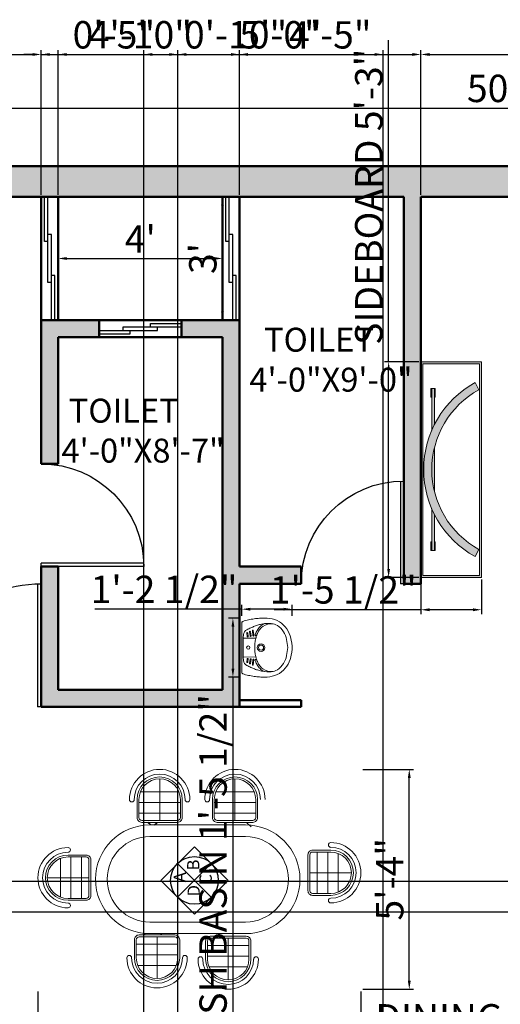
# Model space of a CAD drawing. Units: inches. Extents: x 1770 to 3141, y 984 to 1614.
# Tile 4 of 12: x 1974 to 2115, y 1320 to 1608. Entities that reach past the tile are written whole.
import ezdxf

# ---------------------------------------------------------------- set-up
doc = ezdxf.new("R2010")
doc.units = ezdxf.units.IN
for name, color, linetype, lineweight in [('0.15', 34, 'Continuous', 15), ('A-ANNO-DIMS', 2, 'Continuous', 18), ('A-AREA-IDEN', 3, 'Continuous', 18), ('A-DOOR', 4, 'Continuous', 25), ('A-FLOR-FIXT', 8, 'Continuous', 18), ('A-FURN', 8, 'Continuous', 18), ('A-GLAZ', 5, 'Continuous', 25), ('A-WALL', 7, 'Continuous', 50), ('A-WALL-PATT', 8, 'Continuous', 13), ('aparador', 36, 'Continuous', 9), ('moveis', 254, 'Continuous', 5)]:
    doc.layers.add(name, color=color, linetype=linetype, lineweight=lineweight)
doc.layers.add('4', color=4, linetype='Continuous')
doc.styles.get("Standard").update_dxf_attribs({"font": 'arial.ttf'})
doc.dimstyles.new('ISO-25', dxfattribs={"dimtxt": 8, "dimasz": 2.5, "dimexe": 1.25, "dimexo": 0.625, "dimtad": 1, "dimdec": 1, "dimlunit": 3, "dimtxsty": 'Standard', "dimcen": 2.5, "dimclrt": 1, "dimadec": 0, "dimazin": 0, "dimtfac": 1, "dimtdec": 1, "dimtmove": 0, "dimatfit": 3, "dimfxl": 1, "dimarcsym": 0})

# ---------------------------------------------------------------- blocks, each defined once
blk = doc.blocks.new("D1 3'")
for p, q in [((0, 36), (0, 0)), ((1, 36), (1, 0)), ((0, 0), (1, 0))]:
    blk.add_line(p, q)
blk.add_arc((0, 0), 36, 0, 90)
blk = doc.blocks.new("D2 2'6")
for p, q in [((0, 30), (0, 0)), ((1, 30), (1, 0)), ((0, 0), (1, 0))]:
    blk.add_line(p, q)
blk.add_arc((0, 0), 30, 0, 90)
blk = doc.blocks.new('*D17')
at = {"layer": 'A-ANNO-DIMS', "color": 0, "lineweight": -2, "transparency": 16777216}
for p, q in [((1812.73, 1565.8), (1812.73, 1583.37)), ((1815.23, 1582.12), (2410.23, 1582.12)), ((2412.73, 1565.8), (2412.73, 1583.37))]:
    blk.add_line(p, q, dxfattribs=at)
at = {"layer": 'A-ANNO-DIMS', "color": 0, "transparency": 16777216}
for points in [[(1815.23, 1582.54), (1815.23, 1581.7), (1812.73, 1582.12)], [(2410.23, 1582.54), (2410.23, 1581.7), (2412.73, 1582.12)]]:
    blk.add_solid(points, dxfattribs=at)
at = {"layer": 'Defpoints', "color": 0, "transparency": 16777216}
for p in [(2412.73, 1582.12), (1812.73, 1565.18), (2412.73, 1565.18)]:
    blk.add_point(p, dxfattribs=at)
at = {"layer": 'A-ANNO-DIMS', "color": 0, "transparency": 16777216, "insert": (2112.73, 1586.83), "char_height": 8, "attachment_point": 5}
blk.add_mtext("50'", dxfattribs=at)
blk = doc.blocks.new('A$C124A256F')
for p, q in [((-0.448, 1.309), (-0.448, 0.772)), ((0.523, 1.309), (0.523, 0.772)), ((-0.697, 1.141), (-0.2, 1.141)), ((0.772, 1.141), (0.275, 1.141)), ((-0.715, 1.006), (-0.181, 1.006)), ((0.791, 1.006), (0.256, 1.006)), ((-0.715, 0.867), (-0.181, 0.867)), ((0.791, 0.867), (0.256, 0.867)), ((-1.729, -0.214), (-1.729, 0.283)), ((-1.594, -0.233), (-1.594, 0.302)), ((-1.455, -0.233), (-1.455, 0.302)), ((1.583, -0.169), (1.583, 0.365)), ((1.721, -0.169), (1.721, 0.365)), ((1.856, -0.15), (1.856, 0.346)), ((-1.897, 0.034), (-1.361, 0.034)), ((2.025, 0.098), (1.488, 0.098)), ((-0.482, -1.265), (-0.482, -0.728)), ((0.436, -1.282), (0.436, -0.745)), ((-0.749, -0.823), (-0.215, -0.823)), ((0.704, -0.84), (0.169, -0.84)), ((-0.749, -0.962), (-0.215, -0.962)), ((0.704, -0.978), (0.169, -0.978)), ((-0.73, -1.097), (-0.233, -1.097)), ((0.685, -1.114), (0.188, -1.114))]:
    blk.add_line(p, q)
for points in [[(-0.217, 0.748), (-0.679, 0.748, -0.414214), (-0.74, 0.809), (-0.74, 1.042, -1), (-0.157, 1.042), (-0.157, 0.809, -0.414214)], [(-0.217, 0.772), (-0.679, 0.772, -0.414214), (-0.715, 0.809), (-0.715, 1.042, -1), (-0.181, 1.042), (-0.181, 0.809, -0.414214)], [(0.293, 0.748), (0.754, 0.748, 0.414214), (0.815, 0.809), (0.815, 1.042, 1), (0.232, 1.042), (0.232, 0.809, 0.414214)], [(0.293, 0.772), (0.754, 0.772, 0.414214), (0.791, 0.809), (0.791, 1.042, 1), (0.256, 1.042), (0.256, 0.809, 0.414214)], [(1.464, 0.329), (1.464, -0.133, 0.414214), (1.525, -0.194), (1.758, -0.194, 1), (1.758, 0.39), (1.525, 0.39, 0.414214)], [(-1.336, 0.265), (-1.336, -0.196, -0.414214), (-1.397, -0.257), (-1.63, -0.257, -1), (-1.63, 0.326), (-1.397, 0.326, -0.414214)], [(-1.361, 0.265), (-1.361, -0.196, -0.414214), (-1.397, -0.233), (-1.63, -0.233, -1), (-1.63, 0.302), (-1.397, 0.302, -0.414214)], [(1.488, 0.329), (1.488, -0.133, 0.414214), (1.525, -0.169), (1.758, -0.169, 1), (1.758, 0.365), (1.525, 0.365, 0.414214)], [(-0.251, -0.704), (-0.713, -0.704, 0.414214), (-0.774, -0.765), (-0.774, -0.998, 1), (-0.19, -0.998), (-0.19, -0.765, 0.414214)], [(-0.251, -0.728), (-0.713, -0.728, 0.414214), (-0.749, -0.765), (-0.749, -0.998, 1), (-0.215, -0.998), (-0.215, -0.765, 0.414214)], [(0.205, -0.721), (0.667, -0.721, -0.414214), (0.728, -0.782), (0.728, -1.015, -1), (0.145, -1.015), (0.145, -0.782, -0.414214)], [(0.205, -0.745), (0.667, -0.745, -0.414214), (0.704, -0.782), (0.704, -1.015, -1), (0.169, -1.015), (0.169, -0.782, -0.414214)]]:
    blk.add_lwpolyline(points, format="xyb", close=True)
for points in [[(-0.026, 0.714), (-0.575, 0.714, 1), (-0.575, -0.687), (-0.026, -0.687)], [(-0.026, -0.687), (0.661, -0.687, 1), (0.661, 0.714), (-0.026, 0.714)], [(0.254, 0.564), (-0.575, 0.564, 1), (-0.575, -0.537), (0.306, -0.537)], [(0.306, -0.537), (0.661, -0.537, 1), (0.661, 0.564), (0.254, 0.564)]]:
    blk.add_lwpolyline(points, format="xyb")
for centre, radius, start, end in [((-0.448, 1.042), 0.389, 0, 180), ((0.523, 1.042), 0.389, 0, 180), ((-0.448, 1.042), 0.328, 0, 180), ((0.523, 1.042), 0.328, 0, 180), ((-0.807, 1.042), 0.0304, 180, 0), ((-0.09, 1.042), 0.0304, 180, 0), ((0.165, 1.042), 0.0304, 180, 0), ((-1.63, 0.034), 0.389, 90, 270), ((-1.63, 0.393), 0.0304, 270, 90), ((1.758, 0.456), 0.0304, 90, 270), ((1.758, 0.098), 0.389, 270, 90), ((1.758, 0.098), 0.328, 270, 90), ((-1.63, 0.034), 0.328, 90, 270), ((1.758, -0.26), 0.0304, 90, 270), ((-1.63, -0.324), 0.0304, 270, 90), ((-0.84, -0.998), 0.0304, 0, 180), ((-0.482, -0.998), 0.389, 180, 0), ((-0.482, -0.998), 0.328, 180, 0), ((-0.123, -0.998), 0.0304, 0, 180), ((0.078, -1.015), 0.0304, 0, 180), ((0.436, -1.015), 0.389, 180, 0), ((0.436, -1.015), 0.328, 180, 0), ((0.795, -1.015), 0.0304, 0, 180)]:
    blk.add_arc(centre, radius, start, end)
at = {"layer": '4'}
for p, q in [((-0.566, 0.714), (-0.6, 0.748)), ((-0.513, 0.714), (-0.479, 0.748)), ((0.733, 0.688), (0.673, 0.748)), ((-0.217, -0.217), (0.217, 0.217)), ((-0.217, 0.217), (0.217, -0.217)), ((-0.659, -0.704), (-0.638, -0.684)), ((-0.421, -0.704), (-0.438, -0.687))]:
    blk.add_line(p, q, dxfattribs=at)
blk.add_lwpolyline([(0, -0.434), (-0.434, 0), (0, 0.434), (0.434, 0)], close=True, dxfattribs=at)
blk.add_circle((0, 0), 0.307, dxfattribs=at)
for s, height, p in [('B', 0.158, (0.064, 0.127)), ('A ', 0.1575, (-0.109, -0.025)), ('C', 0.158, (0.224, -0.057)), ('D', 0.158, (0.07, -0.208))]:
    blk.add_text(s, height=height, rotation=90, dxfattribs=at).set_placement(p)
blk = doc.blocks.new('Aparador ORGANICA Formatto')
at = {"layer": 'aparador', "ltscale": 0.3}
h = blk.add_hatch(color=256, dxfattribs=at)
h.dxf.hatch_style = 1
h.set_gradient(color1=(118, 213, 123), color2=(52, 168, 57), one_color=1, tint=0.43, name='INVCURVED')
h.paths.add_polyline_path([(0.8, 0.45), (-0.8, 0.45), (-0.8, 0), (0.8, 0)])
h.paths.add_polyline_path([(0.785, 0.435), (0.785, 0.015), (-0.785, 0.015), (-0.785, 0.435)], flags=16)
h.paths.add_polyline_path([(0.2911, 0.3699), (0.5365, 0.3699), (0.5365, 0.3757), (0.6011, 0.3757), (0.6011, 0.3699), (0.6011, 0.3499), (0.6011, 0.3441), (0.5365, 0.3441), (0.5365, 0.3499), (0.3338, 0.3499, -0.150336), (0.6449, 0.0488), (0.5923, 0.0199, 0.208852), (0.1632, 0.3499), (-0.1632, 0.3499, 0.208852), (-0.5923, 0.0199), (-0.6449, 0.0488, -0.150336), (-0.3338, 0.3499), (-0.5365, 0.3499), (-0.5365, 0.3441), (-0.6011, 0.3441), (-0.6011, 0.3499), (-0.6011, 0.3699), (-0.6011, 0.3757), (-0.5365, 0.3757), (-0.5365, 0.3699), (-0.2911, 0.3699, -0.206106)], flags=0)
h = blk.add_hatch(color=256, dxfattribs=at)
h.dxf.hatch_style = 1
h.set_gradient(color1=(135, 92, 69), color2=(0, 0, 0), one_color=1, name='INVCURVED')
h.paths.add_polyline_path([(-0.6449, 0.0488), (-0.5923, 0.0199, -0.590888), (0.5923, 0.0199), (0.6449, 0.0488, 0.590888)])
h = blk.add_hatch(color=256, dxfattribs=at)
h.dxf.hatch_style = 1
h.set_gradient(color1=(178, 189, 189), one_color=1, tint=1, name='CYLINDER')
h.paths.add_polyline_path([(-0.5365, 0.3757), (-0.6011, 0.3757), (-0.6011, 0.3699), (-0.5365, 0.3699)])
h.paths.add_polyline_path([(-0.5365, 0.3499), (-0.6011, 0.3499), (-0.6011, 0.3441), (-0.5365, 0.3441)])
h = blk.add_hatch(color=256, dxfattribs=at)
h.dxf.hatch_style = 1
h.set_gradient(color1=(118, 213, 123), color2=(31, 101, 35), one_color=1, tint=0.26, name='INVCURVED')
h.paths.add_polyline_path([(-0.2911, 0.3699), (-0.6011, 0.3699), (-0.6011, 0.3499), (-0.3338, 0.3499, -0.015999)])
h = blk.add_hatch(color=256, dxfattribs=at)
h.dxf.hatch_style = 1
h.set_gradient(color1=(118, 213, 123), color2=(31, 101, 35), one_color=1, tint=0.26, name='INVCURVED')
h.paths.add_polyline_path([(-0.1632, 0.3499), (0.1632, 0.3499, 0.122516)])
h = blk.add_hatch(color=256, dxfattribs=at)
h.dxf.hatch_style = 1
h.set_gradient(color1=(118, 213, 123), color2=(31, 101, 35), one_color=1, tint=0.26, name='INVCURVED')
h.paths.add_polyline_path([(0.6011, 0.3699), (0.2911, 0.3699, -0.015999), (0.3338, 0.3499), (0.6011, 0.3499)])
h = blk.add_hatch(color=256, dxfattribs=at)
h.dxf.hatch_style = 1
h.set_gradient(color1=(178, 189, 189), one_color=1, tint=1, name='CYLINDER')
h.paths.add_polyline_path([(0.6011, 0.3757), (0.5365, 0.3757), (0.5365, 0.3699), (0.6011, 0.3699)])
h.paths.add_polyline_path([(0.6011, 0.3499), (0.5365, 0.3499), (0.5365, 0.3441), (0.6011, 0.3441)])
for p, q in [((-0.5923, 0.0199), (-0.6449, 0.0488)), ((0.5923, 0.0199), (0.6449, 0.0488))]:
    blk.add_line(p, q, dxfattribs=at)
for points in [[(-0.6011, 0.3699), (-0.6011, 0.3757), (-0.5365, 0.3757), (-0.5365, 0.3699)], [(0.6011, 0.3699), (0.6011, 0.3757), (0.5365, 0.3757), (0.5365, 0.3699)], [(-0.5365, 0.3499), (-0.5365, 0.3441), (-0.6011, 0.3441), (-0.6011, 0.3499)], [(0.5365, 0.3499), (0.5365, 0.3441), (0.6011, 0.3441), (0.6011, 0.3499)]]:
    blk.add_lwpolyline(points, dxfattribs=at)
for radius in [0.7362, 0.6762]:
    blk.add_arc((0, -0.3063), radius, 28.84335, 151.15665, dxfattribs=at)
at = {"layer": 'moveis', "ltscale": 0.3}
for p, q in [((-0.6011, 0.3699), (-0.6011, 0.3499)), ((-0.2911, 0.3699), (-0.6011, 0.3699)), ((0.2911, 0.3699), (0.6011, 0.3699)), ((0.6011, 0.3699), (0.6011, 0.3499)), ((-0.6011, 0.3499), (-0.3338, 0.3499)), ((-0.1632, 0.3499), (0.1632, 0.3499)), ((0.6011, 0.3499), (0.3338, 0.3499))]:
    blk.add_line(p, q, dxfattribs=at)
for points in [[(-0.8, 0), (0.8, 0), (0.8, 0.45), (-0.8, 0.45)], [(-0.785, 0.015), (0.785, 0.015), (0.785, 0.435), (-0.785, 0.435)]]:
    blk.add_lwpolyline(points, close=True, dxfattribs=at)
blk = doc.blocks.new('*D56')
at = {"layer": 'A-ANNO-DIMS', "color": 0, "lineweight": -2, "transparency": 16777216}
for p, q in [((1985.73, 1538.8), (1985.73, 1539.43)), ((2033.73, 1538.8), (2033.73, 1539.43)), ((1988.23, 1538.18), (2031.23, 1538.18))]:
    blk.add_line(p, q, dxfattribs=at)
at = {"layer": 'A-ANNO-DIMS', "color": 0, "transparency": 16777216}
for points in [[(1988.23, 1538.6), (1988.23, 1537.76), (1985.73, 1538.18)], [(2031.23, 1538.6), (2031.23, 1537.76), (2033.73, 1538.18)]]:
    blk.add_solid(points, dxfattribs=at)
at = {"layer": 'Defpoints', "color": 0, "transparency": 16777216}
for p in [(1985.73, 1538.18), (2033.73, 1538.18), (2033.73, 1538.18)]:
    blk.add_point(p, dxfattribs=at)
at = {"layer": 'A-ANNO-DIMS', "color": 0, "transparency": 16777216, "insert": (2009.73, 1542.8), "char_height": 8, "attachment_point": 5}
blk.add_mtext("4'", dxfattribs=at)
blk = doc.blocks.new('*D57')
at = {"layer": 'A-ANNO-DIMS', "color": 0, "lineweight": -2, "transparency": 16777216}
for p, q in [((2028.55, 1556.18), (2034.98, 1556.18)), ((2033.73, 1553.68), (2033.73, 1522.68)), ((2028.55, 1520.18), (2034.98, 1520.18))]:
    blk.add_line(p, q, dxfattribs=at)
at = {"layer": 'A-ANNO-DIMS', "color": 0, "transparency": 16777216}
for points in [[(2033.32, 1553.68), (2034.15, 1553.68), (2033.73, 1556.18)], [(2033.32, 1522.68), (2034.15, 1522.68), (2033.73, 1520.18)]]:
    blk.add_solid(points, dxfattribs=at)
at = {"layer": 'Defpoints', "color": 0, "transparency": 16777216}
for p in [(2027.93, 1556.18), (2027.93, 1520.18), (2033.73, 1520.18)]:
    blk.add_point(p, dxfattribs=at)
at = {"layer": 'A-ANNO-DIMS', "color": 0, "transparency": 16777216, "insert": (2029.02, 1538.18), "char_height": 8, "attachment_point": 5, "rotation": 90}
blk.add_mtext("3'", dxfattribs=at)
blk = doc.blocks.new('lavamanos 2')
at = {"layer": '0.15'}
for p, q in [((0, 0.2335), (0, -0.2335)), ((-0.1304, 0.11), (-0.1315, 0.11)), ((-0.1127, 0.112), (-0.1067, 0.1581)), ((-0.1037, 0.1109), (-0.0978, 0.157)), ((-0.0857, 0.1085), (-0.0807, 0.1466)), ((-0.0767, 0.1074), (-0.0718, 0.1455)), ((-0.0587, 0.105), (-0.0548, 0.1351)), ((-0.0497, 0.1039), (-0.0458, 0.134)), ((-0.0142, 0.087), (-0.13, 0.086)), ((-0.0142, -0.087), (-0.13, -0.086)), ((-0.1304, -0.11), (-0.1315, -0.11)), ((-0.1127, -0.112), (-0.1067, -0.1581)), ((-0.1037, -0.1109), (-0.0978, -0.157)), ((-0.0857, -0.1085), (-0.0807, -0.1466)), ((-0.0767, -0.1074), (-0.0718, -0.1455)), ((-0.0587, -0.105), (-0.0548, -0.1351)), ((-0.0497, -0.1039), (-0.0458, -0.134))]:
    blk.add_line(p, q, dxfattribs=at)
for centre, radius in [((-0.178, 0), 0.035), ((-0.178, 0), 0.0235), ((-0.06, 0), 0.015)]:
    blk.add_circle(centre, radius, dxfattribs=at)
for centre, radius, start, end in [((-0.2035, -0.0862), 0.3593, 91.20299, 106.42552), ((-0.2208, -0.6855), 0.9585, 86.55138, 89.41308), ((-0.1663, 0.0005), 0.3024, 136.57187, 154.32772), ((-0.2419, 0.0663), 0.2023, 108.1945, 135.36859), ((-0.2422, 0.0655), 0.1638, 121.99295, 150.58892), ((-0.2657, 0.1037), 0.119, 92.47742, 122.14108), ((-0.2765, 0.0677), 0.1528, 57.2491, 95.54005), ((-0.2442, -0.0128), 0.2368, 77.24819, 96.46321), ((-0.2765, 0.0677), 0.1678, 56.87663, 64.99714), ((-0.3662, -0.002), 0.2627, 40.35252, 49.00458), ((-0.2222, 0.0026), 0.2177, 71.98488, 82.01242), ((-0.3662, -0.002), 0.2777, 40.35252, 49.22548), ((-0.2121, -0.5476), 0.8204, 83.12241, 86.5796), ((-0.3103, -0.315), 0.5472, 69.51913, 73.49118), ((-0.2991, -0.2855), 0.5156, 65.23004, 69.53785), ((5.8279, 30.215), 30.5319, 258.77821, 258.87599), ((-0.2784, -0.2408), 0.4663, 60.24131, 65.2382), ((-0.1265, -0.0657), 0.3287, 69.06009, 78.82181), ((-0.0202, 0.212), 0.0314, 54.79491, 69.06009), ((-0.005, 0.2335), 0.005, 0, 54.79491), ((-0.0557, -0.0178), 0.4111, 158.70106, 171.31016), ((-0.1999, 0.0263), 0.2202, 147.11565, 167.44248), ((-0.2374, 0.11), 0.0921, 27.31862, 39.11562), ((-0.3494, 0.0363), 0.2258, 22.33605, 30.8927), ((-0.2374, 0.11), 0.1071, 27.57433, 39.11562), ((-0.3494, 0.0363), 0.2408, 22.19214, 30.78376), ((-1.2664, -0.2389), 1.1824, 16.36313, 17.77674), ((-0.1315, 0.117), 0.007, 197.40991, 270.49494), ((0.1853, 0.1648), 0.325, 192.53887, 196.70718), ((-0.1305, 0.117), 0.007, 270.49494, 17.39527), ((-1.2664, -0.2389), 1.1974, 17.39527, 17.80495), ((-0.1082, 0.1115), 0.0045, 172.61396, 352.61396), ((-0.1022, 0.1575), 0.0045, 352.61396, 172.61396), ((-0.0812, 0.108), 0.0045, 172.61396, 352.61396), ((-0.0763, 0.146), 0.0045, 352.61396, 172.61396), ((-0.0542, 0.1045), 0.0045, 172.61396, 352.61396), ((-0.0503, 0.1345), 0.0045, 352.61396, 172.61396), ((-0.0648, 0.1184), 0.049, 1.58272, 68.62081), ((-2.1477, 0.0009), 2.1352, 359.97535, 3.19009), ((-0.2093, 0.0056), 0.2558, 171.31016, 181.26266), ((-0.2093, -0.0056), 0.2558, 178.73734, 188.68984), ((0.4664, -0.0834), 0.8953, 169.86317, 174.65802), ((0.4664, 0.0834), 0.8953, 185.34198, 190.13683), ((0.3887, 0.121), 0.517, 185.50529, 189.81306), ((-0.7181, -0.0071), 0.5987, 0.67647, 3.82165), ((-0.7181, 0.0071), 0.5987, 356.17835, 359.32353), ((-2.1477, -0.0009), 2.1352, 356.80991, 0.02465), ((-0.0557, 0.0178), 0.4111, 188.68984, 201.29894), ((-0.1999, -0.0263), 0.2202, 192.55752, 212.88435), ((0.1853, -0.1648), 0.325, 163.29282, 167.46113), ((0.3887, -0.1209), 0.517, 170.18694, 174.49471), ((-0.1663, -0.0005), 0.3024, 205.67228, 223.42813), ((-0.2422, -0.0655), 0.1638, 209.41108, 238.00705), ((-0.3662, 0.002), 0.2627, 310.99542, 319.64748), ((-0.3662, 0.002), 0.2777, 310.77452, 319.64748), ((-0.2374, -0.1099), 0.0921, 320.88438, 332.68138), ((-0.3494, -0.0363), 0.2258, 329.1073, 337.66395), ((-0.2374, -0.1099), 0.1071, 320.88438, 332.42567), ((-0.3494, -0.0363), 0.2408, 329.21624, 337.80786), ((-1.2664, 0.2389), 1.1824, 342.22326, 343.63687), ((-0.1315, -0.117), 0.007, 89.50506, 162.59009), ((-0.1305, -0.117), 0.007, 342.60473, 89.50506), ((-1.2664, 0.2389), 1.1974, 342.19505, 342.60473), ((-0.1082, -0.1115), 0.0045, 7.38604, 187.38604), ((-0.1022, -0.1575), 0.0045, 187.38604, 7.38604), ((-0.0812, -0.108), 0.0045, 7.38604, 187.38604), ((-0.2784, 0.2408), 0.4663, 294.7618, 299.75869), ((-0.0763, -0.146), 0.0045, 187.38604, 7.38604), ((-0.0542, -0.1045), 0.0045, 7.38604, 187.38604), ((-0.0503, -0.1345), 0.0045, 187.38604, 7.38604), ((-0.0648, -0.1184), 0.049, 291.37919, 358.41728), ((-0.2419, -0.0663), 0.2023, 224.63141, 251.8055), ((-0.2657, -0.1036), 0.119, 237.85892, 267.52258), ((-0.2035, 0.0862), 0.3593, 253.57448, 268.79701), ((-0.2765, -0.0677), 0.1528, 264.45995, 302.7509), ((-0.2442, 0.0128), 0.2368, 263.53679, 282.75181), ((-0.2208, 0.6855), 0.9585, 270.58692, 273.44862), ((-0.2765, -0.0677), 0.1678, 295.00286, 303.12337), ((-0.2222, -0.0026), 0.2177, 277.98758, 288.01512), ((-0.2121, 0.5476), 0.8204, 273.4204, 276.87759), ((-0.3103, 0.315), 0.5472, 286.50882, 290.48087), ((-0.2991, 0.2855), 0.5156, 290.46215, 294.76996), ((5.8279, -30.215), 30.5319, 101.12401, 101.22179), ((-0.1265, 0.0657), 0.3287, 281.17819, 290.93991), ((-0.0202, -0.212), 0.0314, 290.93991, 305.20509), ((-0.005, -0.2335), 0.005, 305.20509, 0)]:
    blk.add_arc(centre, radius, start, end, dxfattribs=at)
blk = doc.blocks.new('*D92')
at = {"layer": 'A-ANNO-DIMS', "color": 0, "lineweight": -2, "transparency": 16777216}
for p, q in [((1979.79, 1324.09), (1979.79, 1309.31)), ((2074.16, 1324.09), (2074.16, 1309.31)), ((1982.29, 1310.56), (2071.66, 1310.56)), ((2074.16, 1310.56), (2190.7, 1310.56))]:
    blk.add_line(p, q, dxfattribs=at)
at = {"layer": 'A-ANNO-DIMS', "color": 0, "transparency": 16777216}
for points in [[(1982.29, 1310.98), (1982.29, 1310.15), (1979.79, 1310.56)], [(2071.66, 1310.98), (2071.66, 1310.15), (2074.16, 1310.56)]]:
    blk.add_solid(points, dxfattribs=at)
at = {"layer": 'Defpoints', "color": 0, "transparency": 16777216}
for p in [(1979.79, 1324.72), (2074.16, 1324.72), (2074.16, 1310.56)]:
    blk.add_point(p, dxfattribs=at)
at = {"layer": 'A-ANNO-DIMS', "color": 1, "transparency": 16777216, "insert": (2133.68, 1315.32), "char_height": 8, "attachment_point": 5}
blk.add_mtext('DINING SET 7\'-10 1/2"', dxfattribs=at)
blk = doc.blocks.new('*D93')
at = {"layer": 'A-ANNO-DIMS', "color": 0, "lineweight": -2, "transparency": 16777216}
for p, q in [((2074.79, 1388.94), (2089.57, 1388.94)), ((2088.32, 1327.22), (2088.32, 1386.44)), ((2074.79, 1324.72), (2089.57, 1324.72))]:
    blk.add_line(p, q, dxfattribs=at)
at = {"layer": 'A-ANNO-DIMS', "color": 0, "transparency": 16777216}
for points in [[(2087.9, 1386.44), (2088.74, 1386.44), (2088.32, 1388.94)], [(2087.9, 1327.22), (2088.74, 1327.22), (2088.32, 1324.72)]]:
    blk.add_solid(points, dxfattribs=at)
at = {"layer": 'Defpoints', "color": 0, "transparency": 16777216}
for p in [(2074.16, 1388.94), (2088.32, 1388.94), (2074.16, 1324.72)]:
    blk.add_point(p, dxfattribs=at)
at = {"layer": 'A-ANNO-DIMS', "color": 1, "transparency": 16777216, "insert": (2083.63, 1356.83), "char_height": 8, "attachment_point": 5, "rotation": 90}
blk.add_mtext('5\'-4"', dxfattribs=at)
blk = doc.blocks.new('*D96')
at = {"layer": 'A-ANNO-DIMS', "color": 0, "lineweight": -2, "transparency": 16777216}
for p, q in [((2082.28, 1508.01), (2082.28, 1601.92)), ((2091.11, 1508.01), (2081.03, 1508.01)), ((2082.28, 1447.52), (2082.28, 1505.51)), ((2091.11, 1445.02), (2081.03, 1445.02))]:
    blk.add_line(p, q, dxfattribs=at)
at = {"layer": 'A-ANNO-DIMS', "color": 0, "transparency": 16777216}
for points in [[(2081.87, 1505.51), (2082.7, 1505.51), (2082.28, 1508.01)], [(2081.87, 1447.52), (2082.7, 1447.52), (2082.28, 1445.02)]]:
    blk.add_solid(points, dxfattribs=at)
at = {"layer": 'Defpoints', "color": 0, "transparency": 16777216}
for p in [(2082.28, 1508.01), (2091.73, 1508.01), (2091.73, 1445.02)]:
    blk.add_point(p, dxfattribs=at)
at = {"layer": 'A-ANNO-DIMS', "color": 1, "transparency": 16777216, "insert": (2077.52, 1556.22), "char_height": 8, "attachment_point": 5, "rotation": 90}
blk.add_mtext('SIDEBOARD 5\'-3"', dxfattribs=at)
blk = doc.blocks.new('*D97')
at = {"layer": 'A-ANNO-DIMS', "color": 0, "lineweight": -2, "transparency": 16777216}
for p, q in [((2091.73, 1444.39), (2091.73, 1434.32)), ((2109.45, 1444.39), (2109.45, 1434.32)), ((2091.73, 1435.57), (2048.83, 1435.57)), ((2106.95, 1435.57), (2094.23, 1435.57))]:
    blk.add_line(p, q, dxfattribs=at)
at = {"layer": 'A-ANNO-DIMS', "color": 0, "transparency": 16777216}
for points in [[(2094.23, 1435.99), (2094.23, 1435.15), (2091.73, 1435.57)], [(2106.95, 1435.99), (2106.95, 1435.15), (2109.45, 1435.57)]]:
    blk.add_solid(points, dxfattribs=at)
at = {"layer": 'Defpoints', "color": 0, "transparency": 16777216}
for p in [(2091.73, 1445.02), (2109.45, 1445.02), (2091.73, 1435.57)]:
    blk.add_point(p, dxfattribs=at)
at = {"layer": 'A-ANNO-DIMS', "color": 1, "transparency": 16777216, "insert": (2069.03, 1440.33), "char_height": 8, "attachment_point": 5}
blk.add_mtext('1\'-5 1/2"', dxfattribs=at)
blk = doc.blocks.new('*D98')
at = {"layer": 'A-ANNO-DIMS', "color": 0, "lineweight": -2, "transparency": 16777216}
for p, q in [((2038.75, 1433.14), (2035.53, 1433.14)), ((2036.78, 1430.64), (2036.78, 1418.38)), ((2038.75, 1415.88), (2035.53, 1415.88)), ((2036.78, 1415.88), (2036.78, 1298.62))]:
    blk.add_line(p, q, dxfattribs=at)
at = {"layer": 'A-ANNO-DIMS', "color": 0, "transparency": 16777216}
for points in [[(2036.37, 1430.64), (2037.2, 1430.64), (2036.78, 1433.14)], [(2036.37, 1418.38), (2037.2, 1418.38), (2036.78, 1415.88)]]:
    blk.add_solid(points, dxfattribs=at)
at = {"layer": 'Defpoints', "color": 0, "transparency": 16777216}
for p in [(2039.37, 1433.14), (2036.78, 1415.88), (2039.37, 1415.88)]:
    blk.add_point(p, dxfattribs=at)
at = {"layer": 'A-ANNO-DIMS', "color": 1, "transparency": 16777216, "insert": (2032.02, 1356), "char_height": 8, "attachment_point": 5, "rotation": 89.9999}
blk.add_mtext('WASH BASIN 1\'-5 1/2"', dxfattribs=at)
blk = doc.blocks.new('*D99')
at = {"layer": 'A-ANNO-DIMS', "color": 0, "lineweight": -2, "transparency": 16777216}
for p, q in [((2039.37, 1435.73), (1996.47, 1435.73)), ((2039.37, 1433.76), (2039.37, 1436.98)), ((2051.58, 1435.73), (2041.87, 1435.73)), ((2054.08, 1433.76), (2054.08, 1436.98))]:
    blk.add_line(p, q, dxfattribs=at)
at = {"layer": 'A-ANNO-DIMS', "color": 0, "transparency": 16777216}
for points in [[(2041.87, 1436.15), (2041.87, 1435.31), (2039.37, 1435.73)], [(2051.58, 1436.15), (2051.58, 1435.31), (2054.08, 1435.73)]]:
    blk.add_solid(points, dxfattribs=at)
at = {"layer": 'Defpoints', "color": 0, "transparency": 16777216}
for p in [(2039.37, 1435.73), (2039.37, 1433.14), (2054.08, 1433.14)]:
    blk.add_point(p, dxfattribs=at)
at = {"layer": 'A-ANNO-DIMS', "color": 1, "transparency": 16777216, "insert": (2016.67, 1440.49), "char_height": 8, "attachment_point": 5, "rotation": 359.9999}
blk.add_mtext('1\'-2 1/2"', dxfattribs=at)
blk = doc.blocks.new('*D100')
at = {"layer": 'A-ANNO-DIMS', "color": 0, "lineweight": -2, "transparency": 16777216}
for p, q in [((1812.73, 1565.8), (1812.73, 1599.03)), ((1815.23, 1597.78), (1978.23, 1597.78)), ((1980.73, 1556.8), (1980.73, 1599.03))]:
    blk.add_line(p, q, dxfattribs=at)
at = {"layer": 'A-ANNO-DIMS', "color": 0, "transparency": 16777216}
for points in [[(1815.23, 1598.2), (1815.23, 1597.36), (1812.73, 1597.78)], [(1978.23, 1598.2), (1978.23, 1597.36), (1980.73, 1597.78)]]:
    blk.add_solid(points, dxfattribs=at)
at = {"layer": 'Defpoints', "color": 0, "transparency": 16777216}
for p in [(1980.73, 1597.78), (1812.73, 1565.18), (1980.73, 1556.18)]:
    blk.add_point(p, dxfattribs=at)
at = {"layer": 'A-ANNO-DIMS', "color": 1, "transparency": 16777216, "insert": (1896.73, 1602.49), "char_height": 8, "attachment_point": 5}
blk.add_mtext('14\'-0"', dxfattribs=at)
blk = doc.blocks.new('*D101')
at = {"layer": 'A-ANNO-DIMS', "color": 0, "lineweight": -2, "transparency": 16777216}
for p, q in [((1980.73, 1556.8), (1980.73, 1599.03)), ((1983.23, 1597.78), (2036.23, 1597.78)), ((2038.73, 1556.8), (2038.73, 1599.03))]:
    blk.add_line(p, q, dxfattribs=at)
at = {"layer": 'A-ANNO-DIMS', "color": 0, "transparency": 16777216}
for points in [[(1983.23, 1598.2), (1983.23, 1597.36), (1980.73, 1597.78)], [(2036.23, 1598.2), (2036.23, 1597.36), (2038.73, 1597.78)]]:
    blk.add_solid(points, dxfattribs=at)
at = {"layer": 'Defpoints', "color": 0, "transparency": 16777216}
for p in [(2038.73, 1597.78), (1980.73, 1556.18), (2038.73, 1556.18)]:
    blk.add_point(p, dxfattribs=at)
at = {"layer": 'A-ANNO-DIMS', "color": 1, "transparency": 16777216, "insert": (2009.73, 1602.49), "char_height": 8, "attachment_point": 5}
blk.add_mtext('4\'-10"', dxfattribs=at)
blk = doc.blocks.new('*D102')
at = {"layer": 'A-ANNO-DIMS', "color": 0, "lineweight": -2, "transparency": 16777216}
for p, q in [((2038.73, 1556.8), (2038.73, 1599.03)), ((2041.23, 1597.78), (2089.23, 1597.78)), ((2091.73, 1556.8), (2091.73, 1599.03))]:
    blk.add_line(p, q, dxfattribs=at)
at = {"layer": 'A-ANNO-DIMS', "color": 0, "transparency": 16777216}
for points in [[(2041.23, 1598.2), (2041.23, 1597.36), (2038.73, 1597.78)], [(2089.23, 1598.2), (2089.23, 1597.36), (2091.73, 1597.78)]]:
    blk.add_solid(points, dxfattribs=at)
at = {"layer": 'Defpoints', "color": 0, "transparency": 16777216}
for p in [(2091.73, 1597.78), (2038.73, 1556.18), (2091.73, 1556.18)]:
    blk.add_point(p, dxfattribs=at)
at = {"layer": 'A-ANNO-DIMS', "color": 1, "transparency": 16777216, "insert": (2065.23, 1602.47), "char_height": 8, "attachment_point": 5}
blk.add_mtext('4\'-5"', dxfattribs=at)
blk = doc.blocks.new('*D103')
at = {"layer": 'A-ANNO-DIMS', "color": 0, "lineweight": -2, "transparency": 16777216}
for p, q in [((2091.73, 1556.8), (2091.73, 1599.03)), ((2094.23, 1597.78), (2237.23, 1597.78)), ((2239.73, 1565.8), (2239.73, 1599.03))]:
    blk.add_line(p, q, dxfattribs=at)
at = {"layer": 'A-ANNO-DIMS', "color": 0, "transparency": 16777216}
for points in [[(2094.23, 1598.2), (2094.23, 1597.36), (2091.73, 1597.78)], [(2237.23, 1598.2), (2237.23, 1597.36), (2239.73, 1597.78)]]:
    blk.add_solid(points, dxfattribs=at)
at = {"layer": 'Defpoints', "color": 0, "transparency": 16777216}
for p in [(2239.73, 1597.78), (2239.73, 1565.18), (2091.73, 1556.18)]:
    blk.add_point(p, dxfattribs=at)
at = {"layer": 'A-ANNO-DIMS', "color": 1, "transparency": 16777216, "insert": (2165.73, 1602.42), "char_height": 8, "attachment_point": 5}
blk.add_mtext('12\'-4"', dxfattribs=at)
blk = doc.blocks.new('*D106')
at = {"layer": 'A-ANNO-DIMS', "color": 0, "lineweight": -2, "transparency": 16777216}
for p, q in [((1978.23, 1597.78), (1975.73, 1597.78)), ((1980.73, 1556.8), (1980.73, 1599.03)), ((1980.73, 1597.78), (1985.73, 1597.78)), ((1985.73, 1556.8), (1985.73, 1599.03)), ((1988.23, 1597.78), (2013.25, 1597.78))]:
    blk.add_line(p, q, dxfattribs=at)
at = {"layer": 'A-ANNO-DIMS', "color": 0, "transparency": 16777216}
for points in [[(1978.23, 1598.2), (1978.23, 1597.36), (1980.73, 1597.78)], [(1988.23, 1598.2), (1988.23, 1597.36), (1985.73, 1597.78)]]:
    blk.add_solid(points, dxfattribs=at)
at = {"layer": 'Defpoints', "color": 0, "transparency": 16777216}
for p in [(1985.73, 1597.78), (1980.73, 1556.18), (1985.73, 1556.18)]:
    blk.add_point(p, dxfattribs=at)
at = {"layer": 'A-ANNO-DIMS', "color": 1, "transparency": 16777216, "insert": (2001.99, 1602.49), "char_height": 8, "attachment_point": 5}
blk.add_mtext('0\'-5"', dxfattribs=at)
blk = doc.blocks.new('*D116')
at = {"layer": 'A-ANNO-DIMS', "color": 0, "lineweight": -2, "transparency": 16777216}
for p, q in [((2010.73, 1100.8), (2010.73, 1599.03)), ((2013.23, 1597.78), (2018.19, 1597.78)), ((2020.69, 1094.8), (2020.69, 1599.03)), ((2020.69, 1597.78), (2051.92, 1597.78))]:
    blk.add_line(p, q, dxfattribs=at)
at = {"layer": 'A-ANNO-DIMS', "color": 0, "transparency": 16777216}
for points in [[(2013.23, 1598.2), (2013.23, 1597.36), (2010.73, 1597.78)], [(2018.19, 1598.2), (2018.19, 1597.36), (2020.69, 1597.78)]]:
    blk.add_solid(points, dxfattribs=at)
at = {"layer": 'Defpoints', "color": 0, "transparency": 16777216}
for p in [(2020.69, 1597.78), (2010.73, 1100.18), (2020.69, 1094.18)]:
    blk.add_point(p, dxfattribs=at)
at = {"layer": 'A-ANNO-DIMS', "color": 1, "transparency": 16777216, "insert": (2037.56, 1602.49), "char_height": 8, "attachment_point": 5}
blk.add_mtext('0\'-10"', dxfattribs=at)
blk = doc.blocks.new('*D117')
at = {"layer": 'A-ANNO-DIMS', "color": 0, "lineweight": -2, "transparency": 16777216}
for p, q in [((2020.69, 1094.8), (2020.69, 1599.03)), ((2023.19, 1597.78), (2078.19, 1597.78)), ((2080.69, 1094.8), (2080.69, 1599.03))]:
    blk.add_line(p, q, dxfattribs=at)
at = {"layer": 'A-ANNO-DIMS', "color": 0, "transparency": 16777216}
for points in [[(2023.19, 1598.2), (2023.19, 1597.36), (2020.69, 1597.78)], [(2078.19, 1598.2), (2078.19, 1597.36), (2080.69, 1597.78)]]:
    blk.add_solid(points, dxfattribs=at)
at = {"layer": 'Defpoints', "color": 0, "transparency": 16777216}
for p in [(2080.69, 1597.78), (2020.69, 1094.18), (2080.69, 1094.18)]:
    blk.add_point(p, dxfattribs=at)
at = {"layer": 'A-ANNO-DIMS', "color": 1, "transparency": 16777216, "insert": (2050.69, 1602.49), "char_height": 8, "attachment_point": 5}
blk.add_mtext('5\'-0"', dxfattribs=at)
blk = doc.blocks.new('*D120')
at = {"layer": 'A-ANNO-DIMS', "color": 0, "lineweight": -2, "transparency": 16777216}
for p, q in [((2333.11, 1356.18), (1778.88, 1356.18)), ((1780.13, 1353.68), (1780.13, 1349.68)), ((2333.11, 1347.18), (1778.88, 1347.18)), ((1780.13, 1347.18), (1780.13, 1322.16))]:
    blk.add_line(p, q, dxfattribs=at)
at = {"layer": 'A-ANNO-DIMS', "color": 0, "transparency": 16777216}
for points in [[(1779.72, 1353.68), (1780.55, 1353.68), (1780.13, 1356.18)], [(1779.72, 1349.68), (1780.55, 1349.68), (1780.13, 1347.18)]]:
    blk.add_solid(points, dxfattribs=at)
at = {"layer": 'Defpoints', "color": 0, "transparency": 16777216}
for p in [(2333.73, 1356.18), (1780.13, 1347.18), (2333.73, 1347.18)]:
    blk.add_point(p, dxfattribs=at)
at = {"layer": 'A-ANNO-DIMS', "color": 1, "transparency": 16777216, "insert": (1775.42, 1333.42), "char_height": 8, "attachment_point": 5, "rotation": 90}
blk.add_mtext('0\'-9"', dxfattribs=at)

msp = doc.modelspace()

# ---------------------------------------------------------------- hatches: boundary and pattern name
at = {"layer": 'A-WALL-PATT'}
h = msp.add_hatch(color=256, dxfattribs=at)
h.dxf.hatch_style = 1
h.paths.add_polyline_path([(1821.73, 1556.18), (1844.25, 1556.18), (2086.73, 1556.18), (2086.73, 1443.18), (2091.73, 1443.18), (2091.73, 1556.18), (2239.73, 1556.18), (2239.73, 1565.18), (1812.73, 1565.18), (1812.73, 1100.18), (1821.73, 1100.18), (1821.73, 1246.18), (1913.73, 1246.18), (1913.73, 1251.18), (1821.73, 1251.18), (1821.73, 1407.18), (1944.73, 1407.18), (1944.73, 1412.18), (1821.73, 1412.18)])
h.paths.add_polyline_path([(1985.73, 1515.18), (1997.73, 1515.18), (1997.73, 1520.18), (1980.73, 1520.18), (1980.73, 1478.18), (1985.73, 1478.18)], flags=16)
h.paths.add_polyline_path([(2038.73, 1520.18), (2021.73, 1520.18), (2021.73, 1515.18), (2033.73, 1515.18), (2033.73, 1412.18), (1985.73, 1412.18), (1985.73, 1448.18), (1980.73, 1448.18), (1980.73, 1407.18), (2038.73, 1407.18), (2038.73, 1443.18), (2056.73, 1443.18), (2056.73, 1448.18), (2038.73, 1448.18)], flags=17)
h.paths.add_polyline_path([(1853.23, 1094.18), (1821.73, 1094.18), (1821.73, 1085.18), (1853.23, 1085.18)])
h.paths.add_polyline_path([(2001.73, 1094.18), (1966.73, 1094.18), (1966.73, 1124.18), (1961.73, 1124.18), (1961.73, 1094.18), (1889.23, 1094.18), (1889.23, 1085.18), (2001.73, 1085.18)])
h.paths.add_polyline_path([(2020.69, 1094.18), (2010.73, 1094.18), (2010.73, 1085.18), (2020.69, 1085.18)])
h.paths.add_polyline_path([(2116.73, 1094.18), (2080.69, 1094.18), (2080.69, 1085.18), (2116.73, 1085.18)])
h.paths.add_polyline_path([(2125.73, 1184.68), (2116.73, 1184.68), (2116.73, 1159.18), (2056.73, 1159.18), (2056.73, 1246.18), (2086.73, 1246.18), (2086.73, 1251.18), (2001.73, 1251.18), (2001.73, 1246.18), (2051.73, 1246.18), (2051.73, 1159.18), (1966.73, 1159.18), (1966.73, 1246.18), (1971.73, 1246.18), (1971.73, 1251.18), (1961.73, 1251.18), (1961.73, 1154.18), (1991.73, 1154.18), (2125.73, 1154.18)], flags=17)
h.paths.add_polyline_path([(2125.73, 1256.18), (2116.73, 1256.18), (2116.73, 1220.68), (2125.73, 1220.68)], flags=17)
h.paths.add_polyline_path([(2128.73, 1309.18), (2116.73, 1309.18), (2116.73, 1292.18), (2125.73, 1292.18), (2125.73, 1300.18), (2128.73, 1300.18)], flags=17)
h.paths.add_polyline_path([(2239.73, 1309.18), (2217.73, 1309.18), (2217.73, 1300.18), (2239.73, 1300.18)], flags=17)
h.paths.add_polyline_path([(2181.73, 1309.18), (2176.73, 1309.18), (2176.73, 1300.18), (2181.73, 1300.18)], flags=17)

# ---------------------------------------------------------------- linework, layer by layer
at = {"layer": 'A-GLAZ'}
for p, q in [((1981.73, 1543.18), (1981.73, 1556.18)), ((1982.73, 1531.18), (1982.73, 1556.18)), ((2034.73, 1543.18), (2034.73, 1556.18)), ((2035.73, 1531.18), (2035.73, 1556.18)), ((1983.73, 1545.18), (1982.73, 1545.18)), ((1983.73, 1520.18), (1983.73, 1545.18)), ((2036.73, 1545.18), (2035.73, 1545.18)), ((2036.73, 1520.18), (2036.73, 1545.18)), ((1982.73, 1543.18), (1981.73, 1543.18)), ((2035.73, 1543.18), (2034.73, 1543.18)), ((1984.73, 1533.18), (1983.73, 1533.18)), ((1984.73, 1520.18), (1984.73, 1533.18)), ((2037.73, 1533.18), (2036.73, 1533.18)), ((2037.73, 1520.18), (2037.73, 1533.18)), ((1983.73, 1531.18), (1982.73, 1531.18)), ((2036.73, 1531.18), (2035.73, 1531.18)), ((2012.73, 1518.18), (2012.73, 1519.18)), ((2012.73, 1519.18), (2021.73, 1519.18)), ((1997.73, 1517.18), (2014.73, 1517.18)), ((1997.73, 1516.18), (2006.73, 1516.18)), ((2004.73, 1517.18), (2004.73, 1518.18)), ((2004.73, 1518.18), (2021.73, 1518.18)), ((2006.73, 1516.18), (2006.73, 1517.18)), ((2014.73, 1517.18), (2014.73, 1518.18))]:
    msp.add_line(p, q, dxfattribs=at)
at = {"layer": 'A-WALL'}
for p, q in [((1812.73, 1565.18), (2412.73, 1565.18)), ((1821.73, 1556.18), (2086.73, 1556.18)), ((1980.73, 1478.18), (1980.73, 1556.18)), ((1985.73, 1520.18), (1985.73, 1556.18)), ((2033.73, 1520.18), (2033.73, 1556.18)), ((2038.73, 1556.18), (2038.73, 1448.18)), ((2086.73, 1556.18), (2086.73, 1443.18)), ((2091.73, 1556.18), (2091.73, 1443.18)), ((2091.73, 1556.18), (2239.73, 1556.18)), ((1980.73, 1520.18), (2038.73, 1520.18)), ((1997.73, 1520.18), (1997.73, 1515.18)), ((2021.73, 1520.18), (2021.73, 1515.18)), ((1985.73, 1515.18), (2033.73, 1515.18)), ((1985.73, 1478.18), (1985.73, 1515.18)), ((2033.73, 1412.18), (2033.73, 1515.18)), ((1985.73, 1478.18), (1980.73, 1478.18)), ((1980.73, 1407.18), (1980.73, 1448.18)), ((1985.73, 1448.18), (1980.73, 1448.18)), ((1985.73, 1412.18), (1985.73, 1448.18)), ((2038.73, 1448.18), (2056.73, 1448.18)), ((2056.73, 1448.18), (2056.73, 1443.18)), ((2038.73, 1443.18), (2056.73, 1443.18)), ((2038.73, 1443.18), (2038.73, 1407.18)), ((2086.73, 1443.18), (2091.73, 1443.18)), ((1985.73, 1412.18), (2033.73, 1412.18)), ((1980.73, 1407.18), (2056.73, 1407.18)), ((2038.73, 1409.18), (2056.73, 1409.18)), ((2056.73, 1409.18), (2056.73, 1407.18))]:
    msp.add_line(p, q, dxfattribs=at)

# ---------------------------------------------------------------- block references
at = {"layer": 'A-DOOR', "xscale": -1, "rotation": 270}
msp.add_blockref("D2 2'6", (1980.73, 1448.18), dxfattribs=at)
at = {"layer": 'A-DOOR', "xscale": -1}
for name, p in [("D2 2'6", (2086.73, 1443.18)), ("D1 3'", (1980.73, 1407.18))]:
    msp.add_blockref(name, p, dxfattribs=at)
at = {"layer": 'A-FLOR-FIXT', "xscale": 31.61240364394164, "yscale": 31.61240364394164, "zscale": 31.61240364394164, "rotation": 179.99990349049}
msp.add_blockref('lavamanos 2', (2039.37, 1424.51), dxfattribs=at)
at = {"layer": 'A-FURN', "xscale": 39.3701, "yscale": 39.3701, "zscale": 39.3701, "rotation": 90}
msp.add_blockref('Aparador ORGANICA Formatto', (2109.45, 1476.52), dxfattribs=at)
at = {"layer": 'A-FURN', "xscale": 22.65588375884486, "yscale": 22.65588375884486, "zscale": 22.65588375884486}
msp.add_blockref('A$C124A256F', (2025.53, 1356.52), dxfattribs=at)

# ---------------------------------------------------------------- texts
at = {"layer": 'A-AREA-IDEN', "char_height": 7, "attachment_point": 1}
for s, insert in [('  TOILET\\P4\'-0"X9\'-0"', (2041.59, 1517.95)), ('  TOILET\\P 4\'-0"X8\'-7"', (1984.54, 1497.22))]:
    msp.add_mtext_dynamic_manual_height_columns(s, width=86.9528, gutter_width=12.5, heights=[0], dxfattribs=dict(at, insert=insert))

# ---------------------------------------------------------------- dimensions: what is measured, and where the dimension line sits
at = {"layer": 'A-ANNO-DIMS'}
for base, p1, p2, override, picture, middle in [((1980.73, 1597.78), (1812.73, 1565.18), (1980.73, 1556.18), {"dimdec": 1, "dimlfac": 1, "dimrnd": 0, "dimzin": 1, "dimdsep": 46, "dimlunit": 4, "dimfrac": 2}, '*D100', (1896.73, 1602.49)), ((1985.73, 1597.78), (1980.73, 1556.18), (1985.73, 1556.18), {"dimdec": 1, "dimlfac": 1, "dimrnd": 0, "dimzin": 1, "dimdsep": 46, "dimlunit": 4, "dimfrac": 2}, '*D106', (2001.99, 1602.49)), ((2038.73, 1597.78), (1980.73, 1556.18), (2038.73, 1556.18), {"dimdec": 1, "dimlfac": 1, "dimrnd": 0, "dimzin": 1, "dimdsep": 46, "dimlunit": 4, "dimfrac": 2}, '*D101', (2009.73, 1602.49)), ((2020.69, 1597.78), (2010.73, 1100.18), (2020.69, 1094.18), {"dimdec": 1, "dimlfac": 1, "dimrnd": 0, "dimzin": 1, "dimdsep": 46, "dimlunit": 4, "dimfrac": 2}, '*D116', (2037.56, 1602.49)), ((2080.69, 1597.78), (2020.69, 1094.18), (2080.69, 1094.18), {"dimdec": 1, "dimlfac": 1, "dimrnd": 0, "dimzin": 1, "dimdsep": 46, "dimlunit": 4, "dimfrac": 2}, '*D117', (2050.69, 1602.49)), ((2091.73, 1597.78), (2038.73, 1556.18), (2091.73, 1556.18), {"dimdec": 1, "dimlfac": 1, "dimrnd": 0, "dimzin": 1, "dimdsep": 46, "dimlunit": 4, "dimfrac": 2}, '*D102', (2065.23, 1602.47)), ((2239.73, 1597.78), (2091.73, 1556.18), (2239.73, 1565.18), {"dimdec": 1, "dimlfac": 1, "dimrnd": 0, "dimzin": 1, "dimdsep": 46, "dimlunit": 4, "dimfrac": 2}, '*D103', (2165.73, 1602.42)), ((2412.73, 1582.12), (1812.73, 1565.18), (2412.73, 1565.18), {"dimclrd": 0, "dimclre": 0, "dimclrt": 0}, '*D17', (2112.73, 1586.83)), ((2033.73, 1538.18), (1985.73, 1538.18), (2033.73, 1538.18), {"dimclrd": 0, "dimclre": 0, "dimclrt": 0}, '*D56', (2009.73, 1542.8))]:
    dim = msp.add_linear_dim(base=base, p1=p1, p2=p2, dimstyle='ISO-25', override=override, dxfattribs=at)
    dim.commit()
    dim.dimension.update_dxf_attribs({"geometry": picture, "text_midpoint": middle})
for base, p1, p2, angle, text, picture, middle in [((2082.28, 1508.01), (2091.73, 1445.02), (2091.73, 1508.01), 90, 'SIDEBOARD <>', '*D96', (2077.52, 1556.22)), ((2036.78, 1415.88), (2039.37, 1433.14), (2039.37, 1415.88), 269.9999, 'WASH BASIN <>', '*D98', (2032.02, 1356))]:
    dim = msp.add_linear_dim(base=base, p1=p1, p2=p2, angle=angle, text=text, dimstyle='ISO-25', override={"dimdec": 1, "dimrnd": 0, "dimzin": 1, "dimlunit": 4, "dimfrac": 2}, dxfattribs=at)
    dim.commit()
    dim.dimension.update_dxf_attribs({"geometry": picture, "text_midpoint": middle})
for base, p1, p2, angle, override, picture, middle in [((2033.73, 1520.18), (2027.93, 1556.18), (2027.93, 1520.18), 90, {"dimclrd": 0, "dimclre": 0, "dimclrt": 0}, '*D57', (2029.02, 1538.18)), ((2039.37, 1435.73), (2054.08, 1433.14), (2039.37, 1433.14), 179.9999, {"dimdec": 1, "dimrnd": 0, "dimzin": 1, "dimlunit": 4, "dimfrac": 2}, '*D99', (2016.67, 1440.49)), ((2091.73, 1435.57), (2109.45, 1445.02), (2091.73, 1445.02), 180, {"dimdec": 1, "dimrnd": 0, "dimzin": 1, "dimlunit": 4, "dimfrac": 2}, '*D97', (2069.03, 1440.33)), ((2088.32, 1388.94), (2074.16, 1324.72), (2074.16, 1388.94), 90, {"dimdec": 1, "dimrnd": 0, "dimzin": 1, "dimlunit": 4, "dimfrac": 2}, '*D93', (2083.63, 1356.83)), ((1780.13, 1347.18), (2333.73, 1356.18), (2333.73, 1347.18), 90, {"dimdec": 1, "dimlfac": 1, "dimrnd": 0, "dimzin": 1, "dimdsep": 46, "dimlunit": 4, "dimfrac": 2}, '*D120', (1775.42, 1333.42))]:
    dim = msp.add_linear_dim(base=base, p1=p1, p2=p2, angle=angle, dimstyle='ISO-25', override=override, dxfattribs=at)
    dim.commit()
    dim.dimension.update_dxf_attribs({"geometry": picture, "text_midpoint": middle})
dim = msp.add_linear_dim(base=(2074.16, 1310.56), p1=(1979.79, 1324.72), p2=(2074.16, 1324.72), text='DINING SET <>', dimstyle='ISO-25', override={"dimdec": 1, "dimrnd": 0, "dimzin": 1, "dimlunit": 4, "dimfrac": 2}, dxfattribs=at)
dim.commit()
dim.dimension.update_dxf_attribs({"geometry": '*D92', "text_midpoint": (2133.68, 1315.32)})

doc.saveas('drawing.dxf')
